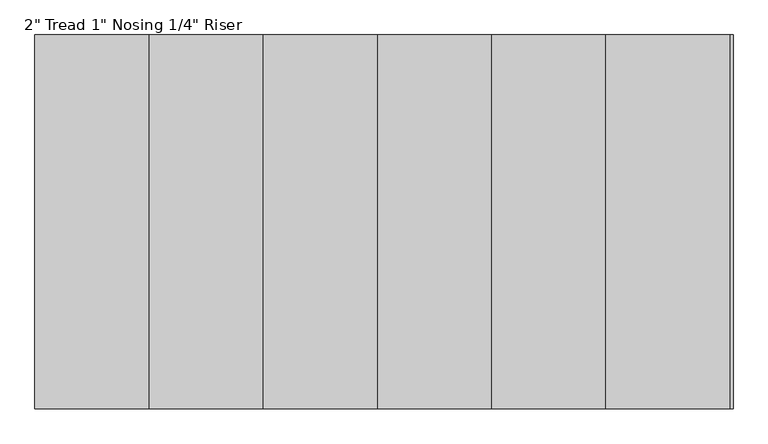
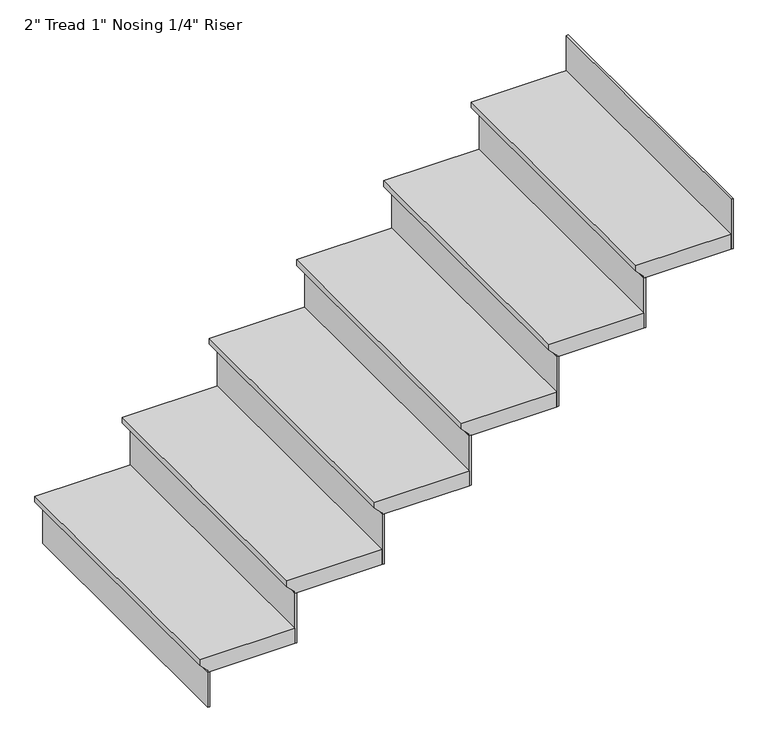
"""IFC4 building model written with IfcOpenShell, lengths in millimetres: stair flight geometry."""

from ifc_helpers import new_model, si_unit, origin, place, context, project, spatial, faceted_brep, source, transform, mapped, element, save


def stair_flight_6437b1f2(model_context):
    return source(origin(), model_context, "Body", "Brep", [
        faceted_brep([(-2479.5608498, 3565.3115866, 3198.2833333), (-2479.5608498, 3565.3115866, 3217.3333333), (-2479.5608498, 4479.7115866, 3217.3333333), (-2479.5608498, 4479.7115866, 3198.2833333), (-2454.1608498, 3565.3115866, 3172.8833333), (-2454.1608498, 4479.7115866, 3172.8833333), (-2174.7608498, 3565.3115866, 3217.3333333), (-2174.7608498, 4479.7115866, 3217.3333333), (-2454.1608498, 4479.7115866, 3166.5333333), (-2174.7608498, 4479.7115866, 3166.5333333), (-2174.7608498, 3565.3115866, 3166.5333333), (-2454.1608498, 3565.3115866, 3166.5333333)], [[[0, 1, 2, 3]], [[4, 0, 3, 5]], [[2, 1, 6, 7]], [[8, 9, 10, 11]], [[2, 7, 9, 8, 5, 3]], [[8, 11, 4, 5]], [[6, 1, 0, 4, 11, 10]], [[7, 6, 10, 9]]]),
        faceted_brep([(-2454.1608498, 3565.3115866, 3166.5333333), (-2454.1608498, 3565.3115866, 3048.0), (-2447.8108498, 3565.3115866, 3048.0), (-2447.8108498, 3565.3115866, 3166.5333333), (-2454.1608498, 4479.7115866, 3166.5333333), (-2447.8108498, 4479.7115866, 3166.5333333), (-2447.8108498, 4479.7115866, 3048.0), (-2454.1608498, 4479.7115866, 3048.0)], [[[0, 1, 2, 3]], [[4, 5, 6, 7]], [[1, 0, 4, 7]], [[2, 1, 7, 6]], [[3, 2, 6, 5]], [[0, 3, 5, 4]]]),
        faceted_brep([(-2174.7608498, 3565.3115866, 3335.8666667), (-2174.7608498, 3565.3115866, 3166.5333333), (-2168.4108498, 3565.3115866, 3166.5333333), (-2168.4108498, 3565.3115866, 3335.8666667), (-2174.7608498, 4479.7115866, 3335.8666667), (-2168.4108498, 4479.7115866, 3335.8666667), (-2168.4108498, 4479.7115866, 3166.5333333), (-2174.7608498, 4479.7115866, 3166.5333333)], [[[0, 1, 2, 3]], [[4, 5, 6, 7]], [[1, 0, 4, 7]], [[2, 1, 7, 6]], [[3, 2, 6, 5]], [[0, 3, 5, 4]]]),
        faceted_brep([(-2200.1608498, 4479.7115866, 3386.6666667), (-2200.1608498, 3565.3115866, 3386.6666667), (-1895.3608498, 3565.3115866, 3386.6666667), (-1895.3608498, 4479.7115866, 3386.6666667), (-2174.7608498, 4479.7115866, 3335.8666667), (-1895.3608498, 4479.7115866, 3335.8666667), (-1895.3608498, 3565.3115866, 3335.8666667), (-2174.7608498, 3565.3115866, 3335.8666667), (-2174.7608498, 4479.7115866, 3342.2166667), (-2200.1608498, 4479.7115866, 3367.6166667), (-2174.7608498, 3565.3115866, 3342.2166667), (-2200.1608498, 3565.3115866, 3367.6166667)], [[[0, 1, 2, 3]], [[4, 5, 6, 7]], [[0, 3, 5, 4, 8, 9]], [[4, 7, 10, 8]], [[2, 1, 11, 10, 7, 6]], [[3, 2, 6, 5]], [[11, 1, 0, 9]], [[10, 11, 9, 8]]]),
        faceted_brep([(-1895.3608498, 3565.3115866, 3505.2), (-1895.3608498, 3565.3115866, 3335.8666667), (-1889.0108498, 3565.3115866, 3335.8666667), (-1889.0108498, 3565.3115866, 3505.2), (-1895.3608498, 4479.7115866, 3505.2), (-1889.0108498, 4479.7115866, 3505.2), (-1889.0108498, 4479.7115866, 3335.8666667), (-1895.3608498, 4479.7115866, 3335.8666667)], [[[0, 1, 2, 3]], [[4, 5, 6, 7]], [[1, 0, 4, 7]], [[2, 1, 7, 6]], [[3, 2, 6, 5]], [[0, 3, 5, 4]]]),
        faceted_brep([(-1920.7608498, 4479.7115866, 3556.0), (-1920.7608498, 3565.3115866, 3556.0), (-1615.9608498, 3565.3115866, 3556.0), (-1615.9608498, 4479.7115866, 3556.0), (-1895.3608498, 4479.7115866, 3505.2), (-1615.9608498, 4479.7115866, 3505.2), (-1615.9608498, 3565.3115866, 3505.2), (-1895.3608498, 3565.3115866, 3505.2), (-1895.3608498, 4479.7115866, 3511.55), (-1920.7608498, 4479.7115866, 3536.95), (-1895.3608498, 3565.3115866, 3511.55), (-1920.7608498, 3565.3115866, 3536.95)], [[[0, 1, 2, 3]], [[4, 5, 6, 7]], [[0, 3, 5, 4, 8, 9]], [[4, 7, 10, 8]], [[2, 1, 11, 10, 7, 6]], [[3, 2, 6, 5]], [[11, 1, 0, 9]], [[10, 11, 9, 8]]]),
        faceted_brep([(-1615.9608498, 3565.3115866, 3674.5333333), (-1615.9608498, 3565.3115866, 3505.2), (-1609.6108498, 3565.3115866, 3505.2), (-1609.6108498, 3565.3115866, 3674.5333333), (-1615.9608498, 4479.7115866, 3674.5333333), (-1609.6108498, 4479.7115866, 3674.5333333), (-1609.6108498, 4479.7115866, 3505.2), (-1615.9608498, 4479.7115866, 3505.2)], [[[0, 1, 2, 3]], [[4, 5, 6, 7]], [[1, 0, 4, 7]], [[2, 1, 7, 6]], [[3, 2, 6, 5]], [[0, 3, 5, 4]]]),
        faceted_brep([(-1641.3608498, 4479.7115866, 3725.3333333), (-1641.3608498, 3565.3115866, 3725.3333333), (-1336.5608498, 3565.3115866, 3725.3333333), (-1336.5608498, 4479.7115866, 3725.3333333), (-1615.9608498, 4479.7115866, 3674.5333333), (-1336.5608498, 4479.7115866, 3674.5333333), (-1336.5608498, 3565.3115866, 3674.5333333), (-1615.9608498, 3565.3115866, 3674.5333333), (-1615.9608498, 4479.7115866, 3680.8833333), (-1641.3608498, 4479.7115866, 3706.2833333), (-1615.9608498, 3565.3115866, 3680.8833333), (-1641.3608498, 3565.3115866, 3706.2833333)], [[[0, 1, 2, 3]], [[4, 5, 6, 7]], [[0, 3, 5, 4, 8, 9]], [[4, 7, 10, 8]], [[2, 1, 11, 10, 7, 6]], [[3, 2, 6, 5]], [[11, 1, 0, 9]], [[10, 11, 9, 8]]]),
        faceted_brep([(-1336.5608498, 3565.3115866, 3843.8666667), (-1336.5608498, 3565.3115866, 3674.5333333), (-1330.2108498, 3565.3115866, 3674.5333333), (-1330.2108498, 3565.3115866, 3843.8666667), (-1336.5608498, 4479.7115866, 3843.8666667), (-1330.2108498, 4479.7115866, 3843.8666667), (-1330.2108498, 4479.7115866, 3674.5333333), (-1336.5608498, 4479.7115866, 3674.5333333)], [[[0, 1, 2, 3]], [[4, 5, 6, 7]], [[1, 0, 4, 7]], [[2, 1, 7, 6]], [[3, 2, 6, 5]], [[0, 3, 5, 4]]]),
        faceted_brep([(-1361.9608498, 4479.7115866, 3894.6666667), (-1361.9608498, 3565.3115866, 3894.6666667), (-1057.1608498, 3565.3115866, 3894.6666667), (-1057.1608498, 4479.7115866, 3894.6666667), (-1336.5608498, 4479.7115866, 3843.8666667), (-1057.1608498, 4479.7115866, 3843.8666667), (-1057.1608498, 3565.3115866, 3843.8666667), (-1336.5608498, 3565.3115866, 3843.8666667), (-1336.5608498, 4479.7115866, 3850.2166667), (-1361.9608498, 4479.7115866, 3875.6166667), (-1336.5608498, 3565.3115866, 3850.2166667), (-1361.9608498, 3565.3115866, 3875.6166667)], [[[0, 1, 2, 3]], [[4, 5, 6, 7]], [[0, 3, 5, 4, 8, 9]], [[4, 7, 10, 8]], [[2, 1, 11, 10, 7, 6]], [[3, 2, 6, 5]], [[11, 1, 0, 9]], [[10, 11, 9, 8]]]),
        faceted_brep([(-777.7608498, 3565.3115866, 4182.5333333), (-777.7608498, 3565.3115866, 4013.2), (-771.4108498, 3565.3115866, 4013.2), (-771.4108498, 3565.3115866, 4182.5333333), (-777.7608498, 4479.7115866, 4182.5333333), (-771.4108498, 4479.7115866, 4182.5333333), (-771.4108498, 4479.7115866, 4013.2), (-777.7608498, 4479.7115866, 4013.2)], [[[0, 1, 2, 3]], [[4, 5, 6, 7]], [[1, 0, 4, 7]], [[2, 1, 7, 6]], [[3, 2, 6, 5]], [[0, 3, 5, 4]]]),
        faceted_brep([(-1057.1608498, 3565.3115866, 4013.2), (-1057.1608498, 3565.3115866, 3843.8666667), (-1050.8108498, 3565.3115866, 3843.8666667), (-1050.8108498, 3565.3115866, 4013.2), (-1057.1608498, 4479.7115866, 4013.2), (-1050.8108498, 4479.7115866, 4013.2), (-1050.8108498, 4479.7115866, 3843.8666667), (-1057.1608498, 4479.7115866, 3843.8666667)], [[[0, 1, 2, 3]], [[4, 5, 6, 7]], [[1, 0, 4, 7]], [[2, 1, 7, 6]], [[3, 2, 6, 5]], [[0, 3, 5, 4]]]),
        faceted_brep([(-777.7608498, 4479.7115866, 4064.0), (-803.1608498, 4479.7115866, 4064.0), (-1082.5608498, 4479.7115866, 4064.0), (-1082.5608498, 3565.3115866, 4064.0), (-777.7608498, 3565.3115866, 4064.0), (-803.1608498, 4479.7115866, 4013.2), (-777.7608498, 4479.7115866, 4013.2), (-777.7608498, 3565.3115866, 4013.2), (-1057.1608498, 3565.3115866, 4013.2), (-1057.1608498, 4479.7115866, 4013.2), (-1057.1608498, 4479.7115866, 4019.55), (-1082.5608498, 4479.7115866, 4044.95), (-1057.1608498, 3565.3115866, 4019.55), (-1082.5608498, 3565.3115866, 4044.95)], [[[0, 1, 2, 3, 4]], [[5, 6, 7, 8, 9]], [[1, 0, 6, 5]], [[2, 1, 5, 9, 10, 11]], [[9, 8, 12, 10]], [[4, 3, 13, 12, 8, 7]], [[0, 4, 7, 6]], [[13, 3, 2, 11]], [[12, 13, 11, 10]]]),
    ])


if __name__ == "__main__":
    model = new_model("IFC4")
    model_context = context("Model", 3, world=origin())
    ifc_project = project(units=[si_unit("LENGTHUNIT", "METRE", prefix="MILLI")], contexts=[model_context])
    site = spatial("IfcSite", under=ifc_project)
    building = spatial("IfcBuilding", under=site)
    placement = place(None, origin())
    stair_flight_shape = stair_flight_6437b1f2(model_context)
    element("IfcStairFlight", 1, ObjectType="2\" Tread 1\" Nosing 1/4\" Riser", at=placement, inside=building, context=model_context, shape_type="MappedRepresentation", body=[
        mapped(stair_flight_shape, transform((0.0, 0.0, 0.0), x_axis=(1.0, 0.0, 0.0), y_axis=(0.0, 1.0, 0.0), z_axis=(0.0, 0.0, 1.0))),
    ])
    save(model, "model.ifc")
